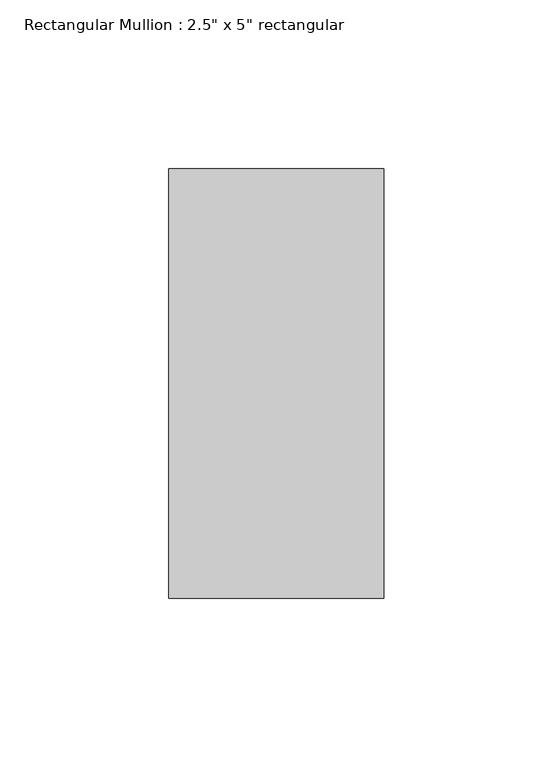
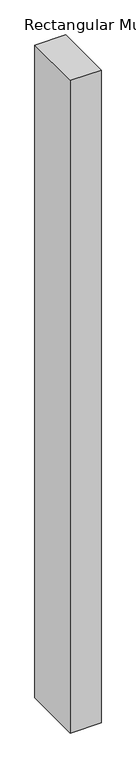
"""IFC4 building model written with IfcOpenShell, lengths in millimetres: member geometry."""

from ifc_helpers import new_model, si_unit, frame, origin, place, context, project, spatial, polyline, outline, extrude, source, transform, mapped, element, save


def member_6df10a9f(model_context):
    return source(origin(), model_context, "Body", "SweptSolid", [
        extrude(outline(polyline([(31.75, 63.5), (31.75, -63.5), (-31.75, -63.5), (-31.75, 63.5), (31.75, 63.5)])), frame((0.0, 0.0, -1428.75), z_axis=(0.0, 0.0, 1.0), x_axis=(1.0, 0.0, 0.0)), (0.0, 0.0, 1.0), 1428.75),
    ])


if __name__ == "__main__":
    model = new_model("IFC4")
    model_context = context("Model", 3, world=origin())
    ifc_project = project(units=[si_unit("LENGTHUNIT", "METRE", prefix="MILLI")], contexts=[model_context])
    site = spatial("IfcSite", under=ifc_project)
    building = spatial("IfcBuilding", under=site)
    placement = place(None, origin())
    member_shape = member_6df10a9f(model_context)
    element("IfcMember", 1, ObjectType="Rectangular Mullion : 2.5\" x 5\" rectangular", at=placement, inside=building, context=model_context, shape_type="MappedRepresentation", body=[
        mapped(member_shape, transform((0.0, 0.0, 0.0), x_axis=(1.0, 0.0, 0.0), y_axis=(0.0, 1.0, 0.0), z_axis=(0.0, 0.0, 1.0))),
    ])
    save(model, "model.ifc")

# Revit data of these elements
# Type "Rectangular Mullion : 2.5\" x 5\" rectangular"
#   built-in parameter 1007304 = 0.416667 (stored number, unit not read)
#   built-in parameter 1007301 = 0.104167 (stored number, unit not read)
#   built-in parameter 1007300 = 0.104167 (stored number, unit not read)
# Element 1 (IfcMember, "Rectangular Mullion : 2.5\" x 5\" rectangular")
#   Materials on its faces: "Aluminum"
# Materials
#   "Aluminum": class "Metal", colour RGB 247 247 247, transparency 0, Description = "Aluminum 6061", Cost = 0
